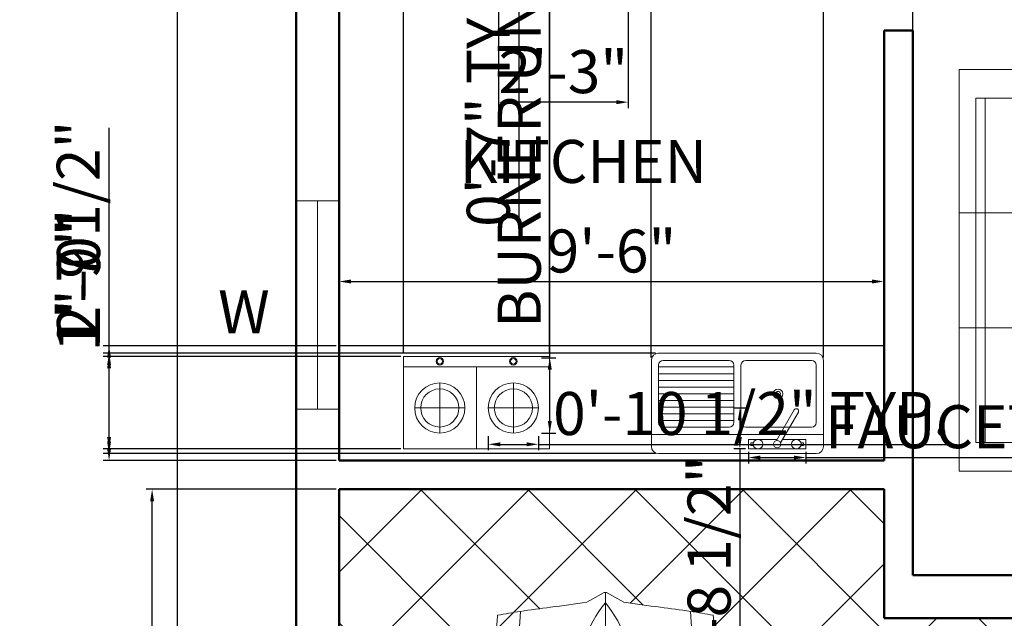
# Model space of a CAD drawing. Units: inches. Extents: x 3587 to 4539, y 1613 to 2440.
# Tile 2 of 8: x 3587 to 3793, y 1803 to 1928. Entities that reach past the tile are written whole.
import ezdxf

# ---------------------------------------------------------------- set-up
doc = ezdxf.new("R2010")
doc.units = ezdxf.units.IN
for name, color, linetype, lineweight in [('A-ANNO-DIMS', 2, 'Continuous', 18), ('A-ANNO-TEXT', 7, 'Continuous', 18), ('A-AREA-IDEN', 7, 'Continuous', 25), ('A-EQPM', 8, 'Continuous', 18), ('A-FLOR-CASE', 32, 'Continuous', 25), ('A-FLOR-FIXT', 9, 'Continuous', 18), ('A-FLOR-PATT', 252, 'Continuous', 13), ('A-FURN', 8, 'Continuous', 18), ('A-GLAZ', 4, 'Continuous', 20), ('A-SITE-VEHI', 9, 'Continuous', 13), ('A-WALL', 7, 'Continuous', 50)]:
    doc.layers.add(name, color=color, linetype=linetype, lineweight=lineweight)
doc.styles.get("Standard").update_dxf_attribs({"font": 'arial.ttf'})
doc.dimstyles.new('ISO-25', dxfattribs={"dimtxt": 9, "dimasz": 2.5, "dimexe": 1.25, "dimexo": 0.625, "dimtad": 1, "dimlunit": 3, "dimtxsty": 'Standard', "dimcen": 2.5, "dimadec": 0, "dimazin": 0, "dimtfac": 1, "dimtmove": 0, "dimatfit": 3, "dimfxl": 1, "dimarcsym": 0})

# ---------------------------------------------------------------- blocks, each defined once
blk = doc.blocks.new('Faucet - kit sink top')
for p, q in [((-5.5, -0.75), (-5.5, -1.25)), ((-4.94278, -0.75), (-5.5, -0.75)), ((-5.5, -1.25), (-4.94278, -1.25)), ((-0.14775, -1.7441), (3.56698, -8.1782)), ((4.43301, -7.6782), (0.71828, -1.2441)), ((4.94278, -0.75), (5.5, -0.75)), ((5.5, -1.25), (4.94278, -1.25)), ((5.5, -0.75), (5.5, -1.25))]:
    blk.add_line(p, q)
blk.add_lwpolyline([(-0.00587, -2), (-6, -2), (-6, 0), (6, 0), (6, -2), (1.15195, -2)])
for centre, radius in [((-4, -1), 1), ((4, -1), 1), ((0, -1), 0.75)]:
    blk.add_circle(centre, radius)
blk.add_arc((4, -7.9282), 0.5, 210, 30)
blk = doc.blocks.new('*U6')
for p, q in [((21.1, 37.41), (21.1, 36.83)), ((46.55, 38.89), (22.35, 38.89)), ((47.8, 37.39), (47.8, 37.41)), ((135.45, 37.07), (135.45, 37.41)), ((136.7, 38.89), (160.9, 38.89)), ((162.15, 37.41), (162.15, 36.77)), ((87.99, 31.87), (74.76, 35.92)), ((134.31, 35.6), (119.29, 31.78)), ((186.47, -33.5), (186.47, 33.5)), ((188.4, -32.76), (188.4, 32.76)), ((70.03, 31.54), (86.41, 29.35)), ((138.42, 29.35), (157.25, 29.35)), ((164.52, 26.39), (164.52, -26.39)), ((186.47, 29.35), (167.01, 29.35)), ((32.27, 11.63), (36.13, 17.17)), ((36.13, 17.17), (50.94, 17.17)), ((32.12, 9.51), (32.12, 11.15)), ((58.92, -10.77), (58.92, 10.77)), ((66.55, -10.53), (66.55, 10.53)), ((186.47, -10.53), (186.47, 10.53)), ((29.77, 9.51), (51.68, 9.51)), ((82.74, 8.5), (82.74, -8.5)), ((3.27, 6.13), (0.1, 0.41)), ((0, 0), (51.68, 0)), ((0.1, -0.41), (3.27, -6.13)), ((29.77, -9.51), (51.68, -9.51)), ((32.12, -9.51), (32.12, -11.15)), ((32.27, -11.63), (36.13, -17.17)), ((36.13, -17.17), (50.94, -17.17)), ((86.41, -29.35), (70.03, -31.54)), ((157.25, -29.35), (138.42, -29.35)), ((167.01, -29.35), (186.47, -29.35)), ((87.99, -31.87), (74.76, -35.92)), ((134.31, -35.6), (119.29, -31.78)), ((21.1, -37.41), (21.1, -36.83)), ((46.55, -38.89), (22.35, -38.89)), ((47.8, -37.39), (47.8, -37.41)), ((135.45, -37.07), (135.45, -37.41)), ((136.7, -38.89), (160.9, -38.89)), ((162.15, -37.41), (162.15, -36.77))]:
    blk.add_line(p, q)
for centre, major_axis, ratio, start_param, end_param in [((41.19, -490.86), (0, 528.23), 0.842304, 0.00281, 0.075598), ((22.35, 37.41), (0, -1.48), 0.842304, 3.141593, 4.712389), ((64.48, -10555.62), (0, 10593.03), 0.842304, -0.013397, 0.002797), ((46.55, 37.41), (0, 1.48), 0.842304, -1.570796, 0), ((136.7, 37.41), (0, -1.48), 0.842304, 3.141593, 4.712389), ((160.9, 37.41), (0, 1.48), 0.842304, -1.570796, 0), ((180.63, 35.84), (0, 2.22), 0.842304, -0.013017, 1.249894), ((64.48, -10556.36), (0, 10595.31), 0.842304, -0.013397, -0.013017), ((183.98, 33.5), (0, -2.96), 0.842304, 1.570796, 3.128196), ((183.98, 32.76), (0, -5.25), 0.842304, 1.570796, 3.128196), ((266.03, -27.52), (0, 313.31), 0.842304, 1.367076, 1.39176), ((64.48, -10555.62), (0, -10591.55), 0.842304, 3.133765, 3.140441), ((37.47, -593.96), (0, -623.33), 0.842304, 3.096046, 3.200911), ((135.29, 5.39), (0, 81.77), 0.842304, 1.245306, 1.50788), ((95.79, -3666.35), (0, -3698.24), 0.842304, 3.134049, 3.144098), ((259.18, -27.52), (0, -305.3), 0.842304, 4.528606, 4.561838), ((134.4, 5.39), (0, -89.78), 0.842304, 4.449482, 4.652344), ((149.6, 2.8), (0, -79.58), 0.842304, 4.372215, 4.640744), ((17.08, 0), (0, 147.02), 0.842304, 4.511394, 4.913384), ((35.91, 0), (0, 147.02), 0.842304, 4.511394, 4.913384), ((167.01, 26.39), (0, 2.96), 0.842304, 0, 1.570796), ((-204.49, 52.4), (0, -250.96), 0.842304, 1.385369, 1.434372), ((13.04, 17.01), (0, 27.42), 0.842304, 4.435146, 4.718221), ((14.2, 17.01), (0, 27.42), 0.842304, 4.435146, 4.718221), ((50.79, 13.34), (6.34, -0.36), 0.603834, -1.395552, 1.581315), ((32.75, 11.15), (0, 0.74), 0.842304, 0.879714, 1.570796), ((29.77, -46.66), (0, 56.17), 0.842304, 0, 0.590319), ((0.62, 0), (0, -0.74), 0.842304, 4.131459, 5.293319), ((29.77, 46.66), (0, 56.17), 0.842304, 2.551274, 3.141593), ((-204.49, -52.4), (0, 250.96), 0.842304, -1.434372, -1.385369), ((13.04, -17.01), (0, -27.42), 0.842304, 1.564964, 1.848039), ((14.2, -17.01), (0, -27.42), 0.842304, 1.564964, 1.848039), ((149.6, -2.8), (0, -79.58), 0.842304, -1.499151, -1.230623), ((32.75, -11.15), (0, -0.74), 0.842304, 4.712389, 5.403472), ((134.4, -5.39), (0, -89.78), 0.842304, -1.510751, -1.307889), ((135.29, -5.39), (0, -81.77), 0.842304, -1.50788, -1.245306), ((259.18, 27.52), (0, 305.3), 0.842304, 1.721348, 1.754579), ((266.03, 27.52), (0, 313.31), 0.842304, 1.749832, 1.774517), ((37.47, 593.96), (0, -623.33), 0.842304, -0.059319, 0.045547), ((167.01, -26.39), (0, -2.96), 0.842304, 4.712389, 6.283185), ((95.79, 3666.35), (0, -3698.24), 0.842304, -0.002505, 0.007544), ((41.19, 490.86), (0, -528.23), 0.842304, -0.075598, -0.00281), ((64.48, 10555.62), (0, -10591.55), 0.842304, 0.001152, 0.007828), ((183.98, -33.5), (0, 2.96), 0.842304, 3.15499, 4.712389), ((183.98, -32.76), (0, -5.25), 0.842304, 0.013397, 1.570796), ((22.35, -37.41), (0, 1.48), 0.842304, 1.570796, 3.141593), ((64.48, 10555.62), (0, 10593.03), 0.842304, 3.138796, 3.15499), ((46.55, -37.41), (0, -1.48), 0.842304, 0, 1.570796), ((136.7, -37.41), (0, -1.48), 0.842304, -1.570796, 0), ((160.9, -37.41), (0, 1.48), 0.842304, 3.141593, 4.712389), ((180.63, -35.84), (0, -2.22), 0.842304, -1.249894, 0.013017), ((64.48, 10556.36), (0, 10595.31), 0.842304, 3.15461, 3.15499)]:
    blk.add_ellipse(centre, major_axis=major_axis, ratio=ratio, start_param=start_param, end_param=end_param)
at = {"extrusion": (0, 0, -1)}
blk.add_ellipse((50.79, -13.34), major_axis=(6.34, 0.36), ratio=0.603834, start_param=-1.395552, end_param=1.581315, dxfattribs=at)
blk = doc.blocks.new('*D14')
at = {"layer": 'A-ANNO-DIMS', "color": 0, "lineweight": -2, "transparency": 16777216}
for p, q in [((3643.9, 2372.93), (3618.39, 2372.93)), ((3619.64, 2370.43), (3619.64, 1655.43)), ((3643.9, 1652.93), (3618.39, 1652.93))]:
    blk.add_line(p, q, dxfattribs=at)
at = {"layer": 'A-ANNO-DIMS', "color": 0, "transparency": 16777216}
for points in [[(3619.22, 2370.43), (3620.05, 2370.43), (3619.64, 2372.93)], [(3619.22, 1655.43), (3620.05, 1655.43), (3619.64, 1652.93)]]:
    blk.add_solid(points, dxfattribs=at)
at = {"layer": 'Defpoints', "color": 0, "transparency": 16777216}
for p in [(3644.52, 2372.93), (3619.64, 1652.93), (3644.52, 1652.93)]:
    blk.add_point(p, dxfattribs=at)
at = {"layer": 'A-ANNO-DIMS', "color": 0, "transparency": 16777216, "insert": (3614.42, 2019.45), "char_height": 9, "attachment_point": 5, "rotation": 90}
blk.add_mtext("60'", dxfattribs=at)
blk = doc.blocks.new('*D25')
at = {"layer": 'A-ANNO-DIMS', "color": 0, "lineweight": -2, "transparency": 16777216}
for p, q in [((3653.52, 1860.56), (3653.52, 1874.64)), ((3767.52, 1860.56), (3767.52, 1874.64)), ((3656.02, 1873.39), (3765.02, 1873.39))]:
    blk.add_line(p, q, dxfattribs=at)
at = {"layer": 'A-ANNO-DIMS', "color": 0, "transparency": 16777216}
for points in [[(3656.02, 1873.81), (3656.02, 1872.98), (3653.52, 1873.39)], [(3765.02, 1873.81), (3765.02, 1872.98), (3767.52, 1873.39)]]:
    blk.add_solid(points, dxfattribs=at)
at = {"layer": 'Defpoints', "color": 0, "transparency": 16777216}
for p in [(3767.52, 1873.39), (3653.52, 1859.93), (3767.52, 1859.93)]:
    blk.add_point(p, dxfattribs=at)
at = {"layer": 'A-ANNO-DIMS', "color": 0, "transparency": 16777216, "insert": (3710.52, 1878.61), "char_height": 9, "attachment_point": 5}
blk.add_mtext('9\'-6"', dxfattribs=at)
blk = doc.blocks.new('*D27')
at = {"layer": 'A-ANNO-DIMS', "color": 0, "lineweight": -2, "transparency": 16777216}
for p, q in [((3773.52, 1812.56), (3773.52, 1940.63)), ((3995.52, 1812.56), (3995.52, 1940.63)), ((3776.02, 1939.38), (3993.02, 1939.38))]:
    blk.add_line(p, q, dxfattribs=at)
at = {"layer": 'A-ANNO-DIMS', "color": 0, "transparency": 16777216}
for points in [[(3776.02, 1939.8), (3776.02, 1938.96), (3773.52, 1939.38)], [(3993.02, 1939.8), (3993.02, 1938.96), (3995.52, 1939.38)]]:
    blk.add_solid(points, dxfattribs=at)
at = {"layer": 'Defpoints', "color": 0, "transparency": 16777216}
for p in [(3995.52, 1939.38), (3773.52, 1811.93), (3995.52, 1811.93)]:
    blk.add_point(p, dxfattribs=at)
at = {"layer": 'A-ANNO-DIMS', "color": 0, "transparency": 16777216, "insert": (3884.52, 1944.6), "char_height": 9, "attachment_point": 5}
blk.add_mtext('18\'-6"', dxfattribs=at)
blk = doc.blocks.new('SOFA-3-SEAT-84IN')
for p, q in [((0, 0), (0, 84)), ((26, 78), (3.47, 78)), ((3.47, 78), (3.47, 6)), ((5.38, 6), (5.38, 78)), ((24.44, 6), (24.44, 78)), ((24.44, 54), (0, 54)), ((24.44, 30), (0, 30)), ((26, 6), (3.47, 6))]:
    blk.add_line(p, q)
for points in [[(0, 84), (26, 84), (26, 78)], [(26, 6), (26, 0), (0, 0)]]:
    blk.add_lwpolyline(points)
blk = doc.blocks.new('WINDOW-43_61IN')
for p, q in [((9, 43.61), (0, 43.61)), ((4.5, 0), (4.5, 43.61)), ((9, 0), (0, 0))]:
    blk.add_line(p, q)
blk = doc.blocks.new('COOKTOP-BURNER-CONTROL')
for p, q in [((5.25, 10.5), (5.25, 0)), ((0, 5.25), (10.5, 5.25))]:
    blk.add_line(p, q)
for centre, radius in [((5.25, 14.99), 0.776), ((5.25, 14.99), 0.571), ((5.25, 5.25), 5.25), ((5.25, 5.25), 3.99)]:
    blk.add_circle(centre, radius)
blk = doc.blocks.new('*D70')
at = {"layer": 'A-ANNO-DIMS', "color": 0, "lineweight": -2, "transparency": 16777216}
for p, q in [((3697.61, 1857.46), (3697.61, 2005.08)), ((3695.87, 1857.46), (3698.86, 1857.46)), ((3697.61, 1844.2), (3697.61, 1854.96)), ((3695.87, 1841.7), (3698.86, 1841.7))]:
    blk.add_line(p, q, dxfattribs=at)
at = {"layer": 'A-ANNO-DIMS', "color": 0, "transparency": 16777216}
for points in [[(3697.19, 1854.96), (3698.02, 1854.96), (3697.61, 1857.46)], [(3697.19, 1844.2), (3698.02, 1844.2), (3697.61, 1841.7)]]:
    blk.add_solid(points, dxfattribs=at)
at = {"layer": 'Defpoints', "color": 0, "transparency": 16777216}
for p in [(3695.24, 1857.46), (3697.61, 1857.46), (3695.24, 1841.7)]:
    blk.add_point(p, dxfattribs=at)
at = {"layer": 'A-ANNO-DIMS', "color": 0, "transparency": 16777216, "insert": (3692.39, 1932.52), "char_height": 9, "attachment_point": 5, "rotation": 90}
blk.add_mtext('BURNER UNIT 1\'-4" TYP.', dxfattribs=at)
blk = doc.blocks.new('*D71')
at = {"layer": 'A-ANNO-DIMS', "color": 0, "lineweight": -2, "transparency": 16777216}
for p, q in [((3684.74, 1841.07), (3684.74, 1838.08)), ((3687.24, 1839.33), (3692.74, 1839.33)), ((3695.24, 1841.07), (3695.24, 1838.08)), ((3695.24, 1839.33), (3781.82, 1839.33))]:
    blk.add_line(p, q, dxfattribs=at)
at = {"layer": 'A-ANNO-DIMS', "color": 0, "transparency": 16777216}
for points in [[(3687.24, 1839.75), (3687.24, 1838.92), (3684.74, 1839.33)], [(3692.74, 1839.75), (3692.74, 1838.92), (3695.24, 1839.33)]]:
    blk.add_solid(points, dxfattribs=at)
at = {"layer": 'Defpoints', "color": 0, "transparency": 16777216}
for p in [(3684.74, 1841.7), (3695.24, 1841.7), (3695.24, 1839.33)]:
    blk.add_point(p, dxfattribs=at)
at = {"layer": 'A-ANNO-DIMS', "color": 0, "transparency": 16777216, "insert": (3739.78, 1844.61), "char_height": 9, "attachment_point": 5}
blk.add_mtext('0\'-10 1/2" TYP.', dxfattribs=at)
blk = doc.blocks.new('*D72')
at = {"layer": 'A-ANNO-DIMS', "color": 0, "lineweight": -2, "transparency": 16777216}
for p, q in [((3739.17, 1837.74), (3739.17, 1835.32)), ((3751.17, 1837.74), (3751.17, 1835.32)), ((3741.67, 1836.57), (3748.67, 1836.57)), ((3751.17, 1836.57), (3832.12, 1836.57))]:
    blk.add_line(p, q, dxfattribs=at)
at = {"layer": 'A-ANNO-DIMS', "color": 0, "transparency": 16777216}
for points in [[(3741.67, 1836.98), (3741.67, 1836.15), (3739.17, 1836.57)], [(3748.67, 1836.98), (3748.67, 1836.15), (3751.17, 1836.57)]]:
    blk.add_solid(points, dxfattribs=at)
at = {"layer": 'Defpoints', "color": 0, "transparency": 16777216}
for p in [(3739.17, 1838.37), (3751.17, 1838.37), (3751.17, 1836.57)]:
    blk.add_point(p, dxfattribs=at)
at = {"layer": 'A-ANNO-DIMS', "color": 0, "transparency": 16777216, "insert": (3792.9, 1841.85), "char_height": 9, "attachment_point": 5}
blk.add_mtext('FAUCET 1\'-0"', dxfattribs=at)
blk = doc.blocks.new('*D73')
at = {"layer": 'A-ANNO-DIMS', "color": 0, "lineweight": -2, "transparency": 16777216}
for p, q in [((3738.55, 1846.87), (3736.12, 1846.87)), ((3737.37, 1844.37), (3737.37, 1840.87)), ((3738.55, 1838.37), (3736.12, 1838.37)), ((3737.37, 1838.37), (3737.37, 1789.72))]:
    blk.add_line(p, q, dxfattribs=at)
at = {"layer": 'A-ANNO-DIMS', "color": 0, "transparency": 16777216}
for points in [[(3736.95, 1844.37), (3737.79, 1844.37), (3737.37, 1846.87)], [(3736.95, 1840.87), (3737.79, 1840.87), (3737.37, 1838.37)]]:
    blk.add_solid(points, dxfattribs=at)
at = {"layer": 'Defpoints', "color": 0, "transparency": 16777216}
for p in [(3739.17, 1846.87), (3737.37, 1838.37), (3739.17, 1838.37)]:
    blk.add_point(p, dxfattribs=at)
at = {"layer": 'A-ANNO-DIMS', "color": 0, "transparency": 16777216, "insert": (3732.09, 1812.79), "char_height": 9, "attachment_point": 5, "rotation": 90}
blk.add_mtext('0\'-8 1/2"', dxfattribs=at)
blk = doc.blocks.new('*D78')
at = {"layer": 'A-ANNO-DIMS', "color": 0, "lineweight": -2, "transparency": 16777216}
for p, q in [((3693.28, 1942.22), (3693.28, 1939.45)), ((3695.78, 1940.7), (3705.1, 1940.7)), ((3707.6, 1942.22), (3707.6, 1939.45)), ((3707.6, 1940.7), (3859.36, 1940.7))]:
    blk.add_line(p, q, dxfattribs=at)
at = {"layer": 'A-ANNO-DIMS', "color": 0, "transparency": 16777216}
for points in [[(3695.78, 1941.11), (3695.78, 1940.28), (3693.28, 1940.7)], [(3705.1, 1941.11), (3705.1, 1940.28), (3707.6, 1940.7)]]:
    blk.add_solid(points, dxfattribs=at)
at = {"layer": 'Defpoints', "color": 0, "transparency": 16777216}
for p in [(3693.28, 1942.85), (3707.6, 1942.85), (3707.6, 1940.7)]:
    blk.add_point(p, dxfattribs=at)
at = {"layer": 'A-ANNO-DIMS', "color": 0, "transparency": 16777216, "insert": (3784.73, 1945.98), "char_height": 9, "attachment_point": 5}
blk.add_mtext('END CHAIR 1\'-2 1/2" TYP.', dxfattribs=at)
blk = doc.blocks.new('*D79')
at = {"layer": 'A-ANNO-DIMS', "color": 0, "lineweight": -2, "transparency": 16777216}
for p, q in [((3692.65, 1950.02), (3689.88, 1950.02)), ((3691.13, 1947.52), (3691.13, 1945.35)), ((3692.65, 1942.85), (3689.88, 1942.85)), ((3691.13, 1942.85), (3691.13, 1884.24))]:
    blk.add_line(p, q, dxfattribs=at)
at = {"layer": 'A-ANNO-DIMS', "color": 0, "transparency": 16777216}
for points in [[(3690.71, 1947.52), (3691.55, 1947.52), (3691.13, 1950.02)], [(3690.71, 1945.35), (3691.55, 1945.35), (3691.13, 1942.85)]]:
    blk.add_solid(points, dxfattribs=at)
at = {"layer": 'Defpoints', "color": 0, "transparency": 16777216}
for p in [(3693.28, 1950.02), (3691.13, 1942.85), (3693.28, 1942.85)]:
    blk.add_point(p, dxfattribs=at)
at = {"layer": 'A-ANNO-DIMS', "color": 0, "transparency": 16777216, "insert": (3685.91, 1912.29), "char_height": 9, "attachment_point": 5, "rotation": 90}
blk.add_mtext('0\'-7" TYP.', dxfattribs=at)
blk = doc.blocks.new('*D85')
at = {"layer": 'A-ANNO-DIMS', "color": 0, "lineweight": -2, "transparency": 16777216}
for p, q in [((3686.85, 1949.39), (3686.85, 1909.67)), ((3714.03, 1949.39), (3714.03, 1909.67)), ((3711.53, 1910.92), (3689.35, 1910.92))]:
    blk.add_line(p, q, dxfattribs=at)
at = {"layer": 'A-ANNO-DIMS', "color": 0, "transparency": 16777216}
for points in [[(3689.35, 1911.33), (3689.35, 1910.5), (3686.85, 1910.92)], [(3711.53, 1911.33), (3711.53, 1910.5), (3714.03, 1910.92)]]:
    blk.add_solid(points, dxfattribs=at)
at = {"layer": 'Defpoints', "color": 0, "transparency": 16777216}
for p in [(3686.85, 1950.02), (3714.03, 1950.02), (3686.85, 1910.92)]:
    blk.add_point(p, dxfattribs=at)
at = {"layer": 'A-ANNO-DIMS', "color": 0, "transparency": 16777216, "insert": (3700.44, 1916.14), "char_height": 9, "attachment_point": 5}
blk.add_mtext('2\'-3"', dxfattribs=at)
blk = doc.blocks.new('*D88')
at = {"layer": 'A-ANNO-DIMS', "color": 0, "lineweight": -2, "transparency": 16777216}
for p, q in [((3605.42, 1859.93), (3605.42, 1887.76)), ((3652.9, 1859.93), (3604.17, 1859.93)), ((3605.42, 1838.43), (3605.42, 1857.43)), ((3652.9, 1835.93), (3604.17, 1835.93))]:
    blk.add_line(p, q, dxfattribs=at)
at = {"layer": 'A-ANNO-DIMS', "color": 0, "transparency": 16777216}
for points in [[(3605.01, 1857.43), (3605.84, 1857.43), (3605.42, 1859.93)], [(3605.01, 1838.43), (3605.84, 1838.43), (3605.42, 1835.93)]]:
    blk.add_solid(points, dxfattribs=at)
at = {"layer": 'Defpoints', "color": 0, "transparency": 16777216}
for p in [(3605.42, 1859.93), (3653.52, 1859.93), (3653.52, 1835.93)]:
    blk.add_point(p, dxfattribs=at)
at = {"layer": 'A-ANNO-DIMS', "color": 0, "transparency": 16777216, "insert": (3600.2, 1875.1), "char_height": 9, "attachment_point": 5, "rotation": 90}
blk.add_mtext('2\'-0"', dxfattribs=at)
blk = doc.blocks.new('*D94')
at = {"layer": 'A-ANNO-DIMS', "color": 0, "lineweight": -2, "transparency": 16777216}
for p, q in [((3652.9, 1829.93), (3613.17, 1829.93)), ((3614.42, 1664.43), (3614.42, 1827.43)), ((3652.9, 1661.93), (3613.17, 1661.93))]:
    blk.add_line(p, q, dxfattribs=at)
at = {"layer": 'A-ANNO-DIMS', "color": 0, "transparency": 16777216}
for points in [[(3614.01, 1827.43), (3614.84, 1827.43), (3614.42, 1829.93)], [(3614.01, 1664.43), (3614.84, 1664.43), (3614.42, 1661.93)]]:
    blk.add_solid(points, dxfattribs=at)
at = {"layer": 'Defpoints', "color": 0, "transparency": 16777216}
for p in [(3614.42, 1829.93), (3653.52, 1829.93), (3653.52, 1661.93)]:
    blk.add_point(p, dxfattribs=at)
at = {"layer": 'A-ANNO-DIMS', "color": 0, "transparency": 16777216, "insert": (3609.2, 1745.93), "char_height": 9, "attachment_point": 5, "rotation": 90}
blk.add_mtext('14\'-0"', dxfattribs=at)
blk = doc.blocks.new('*D96')
at = {"layer": 'A-ANNO-DIMS', "color": 0, "lineweight": -2, "transparency": 16777216}
for p, q in [((3667.04, 1858.35), (3667.04, 2413.28)), ((3669.54, 2412.03), (3695.05, 2412.03)), ((3697.55, 1858.35), (3697.55, 2413.28)), ((3697.55, 2412.03), (3746.35, 2412.03))]:
    blk.add_line(p, q, dxfattribs=at)
at = {"layer": 'A-ANNO-DIMS', "color": 0, "transparency": 16777216}
for points in [[(3669.54, 2412.45), (3669.54, 2411.62), (3667.04, 2412.03)], [(3695.05, 2412.45), (3695.05, 2411.62), (3697.55, 2412.03)]]:
    blk.add_solid(points, dxfattribs=at)
at = {"layer": 'Defpoints', "color": 0, "transparency": 16777216}
for p in [(3697.55, 2412.03), (3667.04, 1857.73), (3697.55, 1857.73)]:
    blk.add_point(p, dxfattribs=at)
at = {"layer": 'A-ANNO-DIMS', "color": 0, "transparency": 16777216, "insert": (3723.2, 2417.31), "char_height": 9, "attachment_point": 5}
blk.add_mtext('2\'-6 1/2"', dxfattribs=at)
blk = doc.blocks.new('*D97')
at = {"layer": 'A-ANNO-DIMS', "color": 0, "lineweight": -2, "transparency": 16777216}
for p, q in [((3605.42, 1857.73), (3605.42, 1905.53)), ((3666.42, 1857.73), (3604.17, 1857.73)), ((3605.42, 1840.86), (3605.42, 1855.23)), ((3666.42, 1838.36), (3604.17, 1838.36))]:
    blk.add_line(p, q, dxfattribs=at)
at = {"layer": 'A-ANNO-DIMS', "color": 0, "transparency": 16777216}
for points in [[(3605.01, 1855.23), (3605.84, 1855.23), (3605.42, 1857.73)], [(3605.01, 1840.86), (3605.84, 1840.86), (3605.42, 1838.36)]]:
    blk.add_solid(points, dxfattribs=at)
at = {"layer": 'Defpoints', "color": 0, "transparency": 16777216}
for p in [(3605.42, 1857.73), (3667.04, 1857.73), (3667.04, 1838.36)]:
    blk.add_point(p, dxfattribs=at)
at = {"layer": 'A-ANNO-DIMS', "color": 0, "transparency": 16777216, "insert": (3600.14, 1882.88), "char_height": 9, "attachment_point": 5, "rotation": 90}
blk.add_mtext('1\'-7 1/2"', dxfattribs=at)
blk = doc.blocks.new('*D98')
at = {"layer": 'A-ANNO-DIMS', "color": 0, "lineweight": -2, "transparency": 16777216}
for p, q in [((3718.85, 1857.52), (3718.85, 2413.28)), ((3721.35, 2412.03), (3752.35, 2412.03)), ((3754.85, 1857.52), (3754.85, 2413.28))]:
    blk.add_line(p, q, dxfattribs=at)
at = {"layer": 'A-ANNO-DIMS', "color": 0, "transparency": 16777216}
for points in [[(3721.35, 2412.45), (3721.35, 2411.62), (3718.85, 2412.03)], [(3752.35, 2412.45), (3752.35, 2411.62), (3754.85, 2412.03)]]:
    blk.add_solid(points, dxfattribs=at)
at = {"layer": 'Defpoints', "color": 0, "transparency": 16777216}
for p in [(3754.85, 2412.03), (3718.85, 1856.9), (3754.85, 1856.9)]:
    blk.add_point(p, dxfattribs=at)
at = {"layer": 'A-ANNO-DIMS', "color": 0, "transparency": 16777216, "insert": (3736.85, 2417.26), "char_height": 9, "attachment_point": 5}
blk.add_mtext('3\'-0"', dxfattribs=at)
blk = doc.blocks.new('*D99')
at = {"layer": 'A-ANNO-DIMS', "color": 0, "lineweight": -2, "transparency": 16777216}
for p, q in [((3605.42, 1858.4), (3605.42, 1885.22)), ((3719.73, 1858.4), (3604.17, 1858.4)), ((3605.42, 1839.9), (3605.42, 1855.9)), ((3719.73, 1837.4), (3604.17, 1837.4))]:
    blk.add_line(p, q, dxfattribs=at)
at = {"layer": 'A-ANNO-DIMS', "color": 0, "transparency": 16777216}
for points in [[(3605.01, 1855.9), (3605.84, 1855.9), (3605.42, 1858.4)], [(3605.01, 1839.9), (3605.84, 1839.9), (3605.42, 1837.4)]]:
    blk.add_solid(points, dxfattribs=at)
at = {"layer": 'Defpoints', "color": 0, "transparency": 16777216}
for p in [(3605.42, 1858.4), (3720.35, 1858.4), (3720.35, 1837.4)]:
    blk.add_point(p, dxfattribs=at)
at = {"layer": 'A-ANNO-DIMS', "color": 0, "transparency": 16777216, "insert": (3600.2, 1873.06), "char_height": 9, "attachment_point": 5, "rotation": 90}
blk.add_mtext('1\'-9"', dxfattribs=at)

msp = doc.modelspace()

# ---------------------------------------------------------------- hatches: boundary and pattern name
at = {"layer": 'A-FLOR-PATT'}
h = msp.add_hatch(dxfattribs=at)
h.set_pattern_fill('ANSI37', color=256, scale=5)
h.paths.add_polyline_path([(3995.523, 1802.933), (3767.523, 1802.933), (3767.523, 1829.933), (3653.523, 1829.933), (3653.523, 1661.933), (3773.523, 1661.933), (3875.78, 1661.933), (3875.78, 1657.433), (3971.78, 1657.433), (3971.78, 1661.933), (3995.523, 1661.933)])
edge = h.paths.add_edge_path(flags=16)
edge.add_ellipse((-2931.215, 1767.797), major_axis=(-6663.992, 0), ratio=0.84230387, start_angle=179.6161332, end_angle=180.0902291, ccw=False)
edge.add_ellipse((3732.777, 1722.366), major_axis=(0.931, 0), ratio=0.8423039, start_angle=0, end_angle=90, ccw=False)
edge.add_line((3733.708, 1722.826), (3733.708, 1706.681))
edge.add_ellipse((3732.777, 1707.14), major_axis=(-0.931, 0), ratio=0.8423039, start_angle=90, end_angle=180, ccw=False)
edge.add_ellipse((-2931.215, 1767.797), major_axis=(-6663.992, 0), ratio=0.84230387, start_angle=179.3813568, end_angle=179.4717285, ccw=False)
edge.add_ellipse((3731.789, 1694.73), major_axis=(1.396, 0), ratio=0.8423039, start_angle=-0.62824, end_angle=68.46476, ccw=False)
edge.add_ellipse((-2931.681, 1767.797), major_axis=(-6665.43, 0), ratio=0.84230387, start_angle=179.3534459, end_angle=179.3717628, ccw=False)
edge.add_ellipse((3729.851, 1692.621), major_axis=(-3.3, 0), ratio=0.8423039, start_angle=90, end_angle=179.35345, ccw=False)
edge.add_line((3729.851, 1689.841), (3688.635, 1689.841))
edge.add_ellipse((3688.635, 1692.621), major_axis=(-3.3, 0), ratio=0.8423039, start_angle=0.64655, end_angle=90, ccw=False)
edge.add_ellipse((10350.167, 1767.797), major_axis=(-6665.43, 0), ratio=0.84230387, start_angle=0.6282372, end_angle=0.6465541, ccw=False)
edge.add_ellipse((3686.698, 1694.73), major_axis=(-1.396, 0), ratio=0.8423039, start_angle=-68.46476, end_angle=0.62824, ccw=False)
edge.add_ellipse((10349.701, 1767.797), major_axis=(-6663.992, 0), ratio=0.84230387, start_angle=0.5282715, end_angle=0.6465541, ccw=False)
edge.add_ellipse((3685.71, 1707.14), major_axis=(-0.931, 0), ratio=0.8423039, start_angle=0, end_angle=90, ccw=False)
edge.add_line((3684.779, 1706.681), (3684.779, 1722.826))
edge.add_ellipse((3685.71, 1722.366), major_axis=(-0.931, 0), ratio=0.8423039, start_angle=-90, end_angle=0, ccw=False)
edge.add_ellipse((10349.701, 1767.797), major_axis=(-6663.992, 0), ratio=0.84230387, start_angle=-0.0902291, end_angle=0.3838668, ccw=False)
edge.add_line((3685.721, 1778.291), (3685.164, 1778.291))
edge.add_ellipse((3685.71, 1779.075), major_axis=(0.931, 0), ratio=0.8423039, start_angle=180, end_angle=270, ccw=False)
edge.add_line((3684.779, 1779.075), (3684.779, 1794.761))
edge.add_ellipse((3685.71, 1794.301), major_axis=(-0.931, 0), ratio=0.8423039, start_angle=-90, end_angle=0, ccw=False)
edge.add_ellipse((4018.041, 1782.449), major_axis=(-332.308, 0), ratio=0.8423039, start_angle=-3.65043, end_angle=-2.17995, ccw=False)
edge.add_ellipse((3726.559, 1641.004), major_axis=(-197.1, 0), ratio=0.8423039, start_angle=-77.87403, end_angle=-76.21947, ccw=False)
edge.add_ellipse((3726.559, 1645.317), major_axis=(192.064, 0), ratio=0.8423039, start_angle=100.20954, end_angle=102.44463, ccw=False)
edge.add_ellipse((3676.281, 1937.008), major_axis=(-157.877, 0), ratio=0.8423039, start_angle=99.25657, end_angle=102.55493)
edge.add_line((3705.388, 1806.307), (3709.243, 1808.439))
edge.add_line((3709.243, 1808.439), (3713.098, 1806.307))
edge.add_ellipse((3742.206, 1937.008), major_axis=(157.877, 0), ratio=0.8423039, start_angle=257.44507, end_angle=260.74343)
edge.add_ellipse((3691.928, 1645.317), major_axis=(192.064, 0), ratio=0.8423039, start_angle=77.55537, end_angle=79.79046, ccw=False)
edge.add_ellipse((3691.928, 1641.004), major_axis=(197.1, 0), ratio=0.8423039, start_angle=76.21947, end_angle=77.87403, ccw=False)
edge.add_ellipse((3400.445, 1782.449), major_axis=(-332.308, 0), ratio=0.8423039, start_angle=182.17995, end_angle=183.65043, ccw=False)
edge.add_ellipse((3732.777, 1794.301), major_axis=(0.931, 0), ratio=0.8423039, start_angle=0, end_angle=90, ccw=False)
edge.add_line((3733.708, 1794.761), (3733.708, 1778.616))
edge.add_ellipse((3732.777, 1779.075), major_axis=(-0.931, 0), ratio=0.8423039, start_angle=90, end_angle=180, ccw=False)
edge = h.paths.add_edge_path(flags=0)
edge.add_ellipse((-2931.215, 1767.797), major_axis=(6663.061, 0), ratio=0.84230387, start_angle=-0.3777642, end_angle=-0.0555943, ccw=False)
edge.add_line((3731.642, 1723.866), (3729.234, 1733.318))
edge.add_ellipse((1402.768, 1748.102), major_axis=(2326.532, 0), ratio=0.84230387, start_angle=-0.364076, end_angle=0.120897)
edge.add_line((3729.293, 1753.011), (3731.841, 1761.332))
edge = h.paths.add_edge_path(flags=0)
edge.add_line((3729.082, 1764.306), (3727.708, 1754.004))
edge.add_ellipse((3711.004, 1714.253), major_axis=(-50.063, 0), ratio=0.8423039, start_angle=247.20809, end_angle=265.12993)
edge.add_line((3714.588, 1756.313), (3703.898, 1756.313))
edge.add_ellipse((3707.482, 1714.253), major_axis=(50.063, 0), ratio=0.8423039, start_angle=94.87007, end_angle=112.79191)
edge.add_line((3690.778, 1754.004), (3689.404, 1764.306))
edge.add_ellipse((3705.854, 1723.251), major_axis=(-51.443, 0), ratio=0.8423039, start_angle=-85.72258, end_angle=-68.16505, ccw=False)
edge.add_line((3702.619, 1766.496), (3715.867, 1766.496))
edge.add_ellipse((3712.632, 1723.251), major_axis=(-51.443, 0), ratio=0.8423039, start_angle=248.16505, end_angle=265.72258, ccw=False)
edge = h.paths.add_edge_path(flags=0)
edge.add_ellipse((3717.634, 1776.41), major_axis=(0.224, 3.988), ratio=0.6038336, start_angle=106.34259, end_angle=270.99799, ccw=False)
edge.add_line((3715.223, 1775.848), (3715.223, 1789.632))
edge.add_ellipse((3679.888, 1789.632), major_axis=(-35.335, 0), ratio=0.8423039, start_angle=180, end_angle=209.43857)
edge.add_ellipse((3738.598, 1789.632), major_axis=(35.335, 0), ratio=0.8423039, start_angle=150.56143, end_angle=180)
edge.add_line((3703.263, 1789.632), (3703.263, 1775.848))
edge.add_ellipse((3700.852, 1776.41), major_axis=(-0.224, 3.988), ratio=0.6038336, start_angle=89.00201, end_angle=253.65741, ccw=False)
edge.add_line((3698.442, 1776.317), (3698.442, 1785.634))
edge.add_line((3698.442, 1785.634), (3702.059, 1788.154))
edge.add_line((3702.059, 1788.154), (3703.263, 1788.154))
edge.add_line((3703.263, 1788.154), (3703.263, 1789.632))
edge.add_ellipse((3738.598, 1789.632), major_axis=(35.335, 0), ratio=0.8423039, start_angle=150.56143, end_angle=180, ccw=False)
edge.add_ellipse((3679.888, 1789.632), major_axis=(-35.335, 0), ratio=0.8423039, start_angle=180, end_angle=209.43857, ccw=False)
edge.add_line((3715.223, 1789.632), (3715.223, 1788.154))
edge.add_line((3715.223, 1788.154), (3716.427, 1788.154))
edge.add_line((3716.427, 1788.154), (3720.044, 1785.634))
edge.add_line((3720.044, 1785.634), (3720.044, 1776.317))
edge = h.paths.add_edge_path(flags=0)
edge.add_line((3727.708, 1721.281), (3727.708, 1709.439))
edge.add_ellipse((3709.243, 1785.774), major_axis=(92.488, 0), ratio=0.8423039, start_angle=256.40187, end_angle=283.59813, ccw=False)
edge.add_line((3690.778, 1709.439), (3690.778, 1721.281))
edge.add_ellipse((3709.243, 1797.616), major_axis=(92.488, 0), ratio=0.8423039, start_angle=256.40187, end_angle=283.59813)
edge = h.paths.add_edge_path(flags=0)
edge.add_line((3727.708, 1703.298), (3727.708, 1691.053))
edge.add_line((3727.708, 1691.053), (3690.778, 1691.053))
edge.add_line((3690.778, 1691.053), (3690.778, 1703.298))
edge.add_ellipse((3692.64, 1703.298), major_axis=(1.862, 0), ratio=0.8423039, start_angle=90, end_angle=180, ccw=False)
edge.add_line((3692.64, 1704.866), (3725.846, 1704.866))
edge.add_ellipse((3725.846, 1703.298), major_axis=(1.862, 0), ratio=0.8423039, start_angle=0, end_angle=90, ccw=False)
edge = h.paths.add_edge_path(flags=0)
edge.add_ellipse((6015.718, 1748.102), major_axis=(2326.532, 0), ratio=0.84230387, start_angle=179.879103, end_angle=180.364076)
edge.add_line((3689.252, 1733.318), (3686.845, 1723.866))
edge.add_ellipse((10349.701, 1767.797), major_axis=(6663.061, 0), ratio=0.84230387, start_angle=180.0555943, end_angle=180.3777642, ccw=False)
edge.add_line((3686.645, 1761.332), (3689.193, 1753.011))
h.paths.add_polyline_path([(3795.361, 1720.017), (3924.21, 1720.017), (3924.21, 1738.563), (3795.361, 1738.563)], flags=24)

# ---------------------------------------------------------------- linework, layer by layer
at = {"layer": 'A-EQPM'}
for p, q in [((3667.042, 1855.532), (3697.551, 1855.532)), ((3682.297, 1855.532), (3682.297, 1838.363))]:
    msp.add_line(p, q, dxfattribs=at)
msp.add_lwpolyline([(3667.042, 1857.729), (3697.551, 1857.729), (3697.551, 1838.363), (3667.042, 1838.363)], close=True, dxfattribs=at)
at = {"layer": 'A-FLOR-CASE'}
msp.add_line((3767.523, 1859.933), (3653.523, 1859.933), dxfattribs=at)
at = {"layer": 'A-FLOR-FIXT'}
for p, q in [((3736.104, 1855.898), (3736.104, 1843.898)), ((3737.604, 1843.898), (3737.604, 1855.898)), ((3718.854, 1841.398), (3754.854, 1841.398))]:
    msp.add_line(p, q, dxfattribs=at)
for points in [[(3753.354, 1858.398), (3720.354, 1858.398)], [(3718.854, 1856.898), (3718.854, 1838.898)], [(3720.354, 1855.898), (3720.354, 1843.898)], [(3735.104, 1856.898), (3721.354, 1856.898)], [(3752.354, 1856.898), (3738.604, 1856.898)], [(3753.354, 1843.898), (3753.354, 1855.898)], [(3754.854, 1838.898), (3754.854, 1856.898)], [(3720.354, 1855.514), (3736.104, 1855.514)], [(3720.354, 1854.112), (3736.104, 1854.112)], [(3720.354, 1852.71), (3736.104, 1852.71)], [(3720.354, 1851.308), (3736.104, 1851.308)], [(3720.354, 1849.907), (3736.104, 1849.907)], [(3720.354, 1848.505), (3736.104, 1848.505)], [(3720.354, 1847.103), (3736.104, 1847.103)], [(3720.354, 1845.701), (3736.104, 1845.701)], [(3720.354, 1844.299), (3736.104, 1844.299)], [(3721.354, 1842.898), (3735.104, 1842.898)], [(3738.604, 1842.898), (3752.354, 1842.898)], [(3720.354, 1837.398), (3753.354, 1837.398)]]:
    msp.add_lwpolyline(points, dxfattribs=at)
for radius in [1, 0.5]:
    msp.add_circle((3745.354, 1849.898), radius, dxfattribs=at)
for centre, radius, start, end in [((3720.354, 1856.898), 1.5, 90, 180), ((3753.354, 1856.898), 1.5, 0, 90), ((3721.354, 1855.898), 1, 90, 180), ((3735.104, 1855.898), 1, 0, 90), ((3738.604, 1855.898), 1, 90, 180), ((3752.354, 1855.898), 1, 0, 90), ((3721.354, 1843.898), 1, 180, 270), ((3735.104, 1843.898), 1, 270, 0), ((3738.604, 1843.898), 1, 180, 270), ((3752.354, 1843.898), 1, 270, 0), ((3720.354, 1838.898), 1.5, 180, 270), ((3753.354, 1838.898), 1.5, 270, 0)]:
    msp.add_arc(centre, radius, start, end, dxfattribs=at)
at = {"layer": 'A-WALL'}
for p, q in [((3644.523, 2372.933), (3644.523, 1652.933)), ((3653.523, 2051.933), (3653.523, 1835.933)), ((3767.523, 1925.933), (3767.523, 1835.933)), ((3773.523, 1925.933), (3767.523, 1925.933)), ((3773.523, 1925.933), (3773.523, 1811.933)), ((3767.523, 1835.933), (3653.523, 1835.933)), ((3767.523, 1829.933), (3653.523, 1829.933)), ((3653.523, 1829.933), (3653.523, 1661.933)), ((3767.523, 1829.933), (3767.523, 1802.933)), ((3947.532, 1811.933), (3773.523, 1811.933)), ((3995.523, 1802.933), (3767.523, 1802.933))]:
    msp.add_line(p, q, dxfattribs=at)

# ---------------------------------------------------------------- block references
at = {"layer": 'A-EQPM'}
for p in [(3669.349, 1841.696), (3684.741, 1841.696)]:
    msp.add_blockref('COOKTOP-BURNER-CONTROL', p, dxfattribs=at)
at = {"layer": 'A-FLOR-FIXT', "xscale": -1, "rotation": 180}
msp.add_blockref('Faucet - kit sink top', (3745.171, 1838.367), dxfattribs=at)
at = {"layer": 'A-FURN'}
msp.add_blockref('SOFA-3-SEAT-84IN', (3783.277, 1833.732), dxfattribs=at)
at = {"layer": 'A-GLAZ'}
msp.add_blockref('WINDOW-43_61IN', (3644.523, 1846.661), dxfattribs=at)
at = {"layer": 'A-SITE-VEHI', "xscale": 0.6290923427641268, "yscale": 0.6290923427641268, "zscale": 0.6290923427641268, "rotation": 270}
msp.add_blockref('*U6', (3709.243, 1808.362), dxfattribs=at)

# ---------------------------------------------------------------- texts
at = {"layer": 'A-ANNO-TEXT', "insert": (3628.233, 1871.518), "char_height": 9, "attachment_point": 1}
msp.add_mtext_dynamic_manual_height_columns('W', width=47.85632, gutter_width=12.5, heights=[0], dxfattribs=at)
at = {"layer": 'A-AREA-IDEN', "insert": (3678.746, 1903.016), "char_height": 9, "attachment_point": 1}
msp.add_mtext_dynamic_manual_height_columns('KITCHEN', width=166.54002, gutter_width=12.5, heights=[0], dxfattribs=at)

# ---------------------------------------------------------------- dimensions: what is measured, and where the dimension line sits
at = {"layer": 'A-ANNO-DIMS'}
for base, p1, p2, override, picture, middle in [((3697.551, 2412.033), (3667.042, 1857.729), (3697.551, 1857.729), {"dimdec": 1, "dimlfac": 1, "dimrnd": 0, "dimzin": 1, "dimdsep": 46, "dimlunit": 4, "dimfrac": 2}, '*D96', (3723.2, 2417.312)), ((3754.854, 2412.033), (3718.854, 1856.898), (3754.854, 1856.898), {"dimdec": 1, "dimlfac": 1, "dimrnd": 0, "dimzin": 1, "dimdsep": 46, "dimlunit": 4, "dimfrac": 2}, '*D98', (3736.854, 2417.256)), ((3995.523, 1939.381), (3773.523, 1811.933), (3995.523, 1811.933), {"dimclrd": 0, "dimclre": 0, "dimclrt": 0}, '*D27', (3884.523, 1944.601)), ((3767.523, 1873.394), (3653.523, 1859.933), (3767.523, 1859.933), {"dimclrd": 0, "dimclre": 0, "dimclrt": 0}, '*D25', (3710.523, 1878.614))]:
    dim = msp.add_linear_dim(base=base, p1=p1, p2=p2, dimstyle='ISO-25', override=override, dxfattribs=at)
    dim.commit()
    dim.dimension.update_dxf_attribs({"geometry": picture, "text_midpoint": middle})
dim = msp.add_linear_dim(base=(3619.637, 1652.933), p1=(3644.523, 2372.933), p2=(3644.523, 1652.933), angle=90, dimstyle='ISO-25', override={"dimclrd": 0, "dimclre": 0, "dimclrt": 0}, dxfattribs=at)
dim.commit()
dim.dimension.update_dxf_attribs({"geometry": '*D14', "text_midpoint": (3619.637, 2019.453), "dimtype": 160})
for base, p1, p2, angle, text, picture, middle in [((3697.608, 1857.458), (3695.244, 1841.696), (3695.244, 1857.458), 90, 'BURNER UNIT <> TYP.', '*D70', (3692.388, 1932.518)), ((3691.13, 1942.846), (3693.278, 1950.019), (3693.278, 1942.846), 270, '<> TYP.', '*D79', (3685.91, 1912.291))]:
    dim = msp.add_linear_dim(base=base, p1=p1, p2=p2, angle=angle, text=text, dimstyle='ISO-25', override={"dimdec": 1, "dimlfac": 1, "dimrnd": 0, "dimzin": 1, "dimdsep": 46, "dimlunit": 4, "dimfrac": 2}, dxfattribs=at)
    dim.commit()
    dim.dimension.update_dxf_attribs({"geometry": picture, "text_midpoint": middle})
for base, p1, p2, text, picture, middle in [((3707.598, 1940.698), (3693.278, 1942.846), (3707.598, 1942.846), 'END CHAIR <> TYP.', '*D78', (3784.728, 1945.976)), ((3695.244, 1839.332), (3684.741, 1841.696), (3695.244, 1841.696), '<> TYP.', '*D71', (3739.78, 1844.61)), ((3751.171, 1836.567), (3739.171, 1838.367), (3751.171, 1838.367), 'FAUCET <>', '*D72', (3792.896, 1841.846))]:
    dim = msp.add_linear_dim(base=base, p1=p1, p2=p2, text=text, dimstyle='ISO-25', override={"dimdec": 1, "dimlfac": 1, "dimrnd": 0, "dimzin": 1, "dimdsep": 46, "dimlunit": 4, "dimfrac": 2}, dxfattribs=at)
    dim.commit()
    dim.dimension.update_dxf_attribs({"geometry": picture, "text_midpoint": middle})
for base, p1, p2, angle, picture, middle in [((3686.85, 1910.917), (3714.027, 1950.017), (3686.85, 1950.017), 180, '*D85', (3700.439, 1916.14)), ((3605.423, 1857.729), (3667.042, 1838.363), (3667.042, 1857.729), 90, '*D97', (3600.145, 1882.879)), ((3605.423, 1859.933), (3653.523, 1835.933), (3653.523, 1859.933), 90, '*D88', (3600.203, 1875.097)), ((3605.423, 1858.398), (3720.354, 1837.398), (3720.354, 1858.398), 90, '*D99', (3600.203, 1873.061)), ((3737.371, 1838.367), (3739.171, 1846.867), (3739.171, 1838.367), 270, '*D73', (3732.092, 1812.795)), ((3614.423, 1829.933), (3653.523, 1661.933), (3653.523, 1829.933), 90, '*D94', (3609.203, 1745.933))]:
    dim = msp.add_linear_dim(base=base, p1=p1, p2=p2, angle=angle, dimstyle='ISO-25', override={"dimdec": 1, "dimlfac": 1, "dimrnd": 0, "dimzin": 1, "dimdsep": 46, "dimlunit": 4, "dimfrac": 2}, dxfattribs=at)
    dim.commit()
    dim.dimension.update_dxf_attribs({"geometry": picture, "text_midpoint": middle})

doc.saveas('drawing.dxf')
